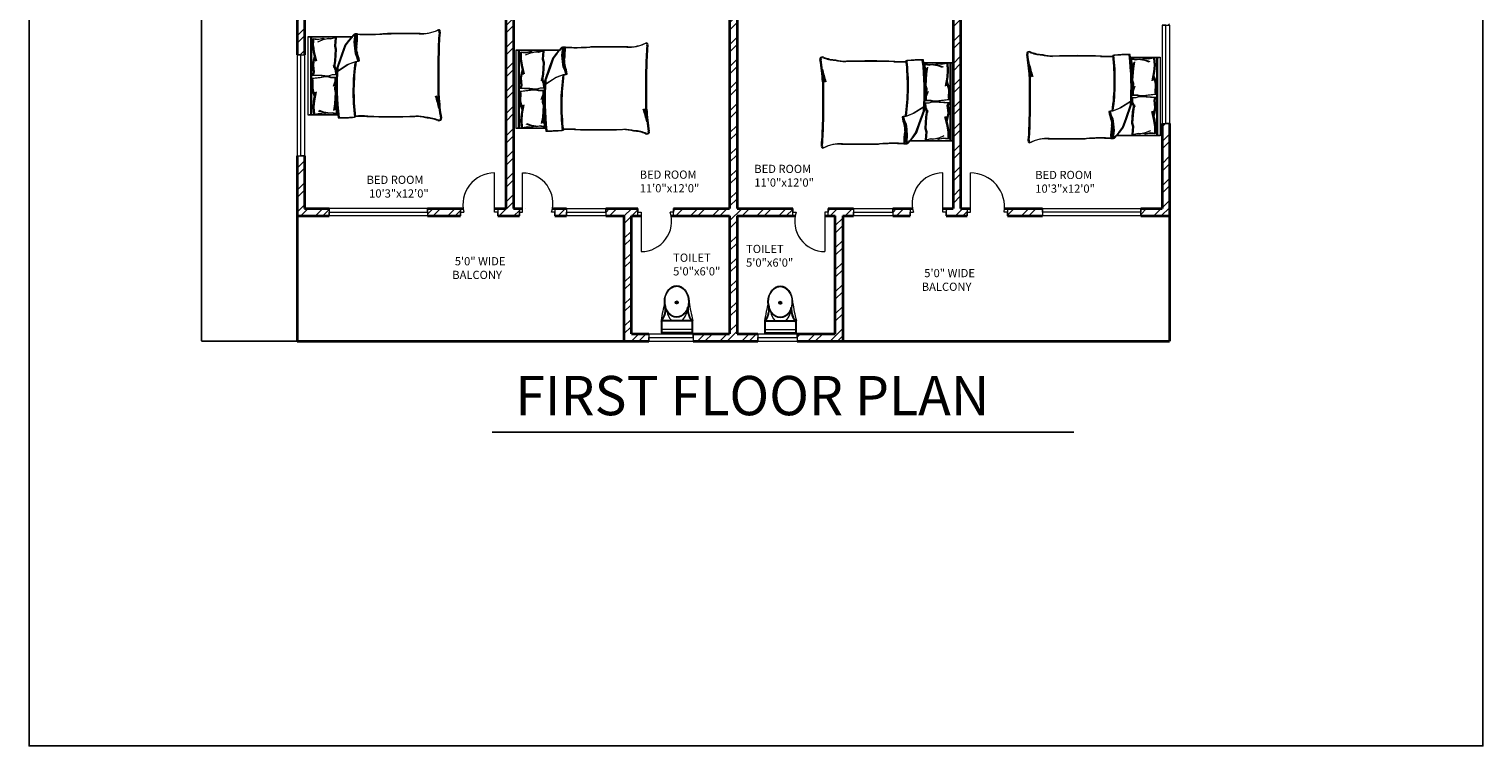
# Model space of a CAD drawing. Units: inches. Extents: x 2168 to 3056, y 1130 to 2629.
# Tile 1 of 42: x 2168 to 3056, y 1130 to 1568. Entities that reach past the tile are written whole.
import ezdxf

# ---------------------------------------------------------------- set-up
doc = ezdxf.new("R2010")
doc.units = ezdxf.units.IN
for name, color, linetype, lineweight in [('A-ANNO-DIMS', 2, 'Continuous', 18), ('A-ANNO-TTLB', 7, 'Continuous', 25), ('A-AREA-IDEN', 7, 'Continuous', 18), ('A-DOOR', 21, 'Continuous', 18), ('A-FLOR-FIXT', 9, 'Continuous', 18), ('A-FURN', 8, 'Continuous', 13), ('A-GLAZ', 201, 'Continuous', 18), ('A-WALL', 7, 'Continuous', 35)]:
    doc.layers.add(name, color=color, linetype=linetype, lineweight=lineweight)
doc.layers.add('A-WALL-PATT', color=143, linetype='Continuous', lineweight=13, true_color=0x7aafdf)
doc.styles.get("Standard").update_dxf_attribs({"font": 'arial.ttf'})
doc.dimstyles.get("Standard").update_dxf_attribs({"dimtxt": 0.18, "dimasz": 0.18, "dimexe": 0.18, "dimexo": 0.0625, "dimgap": 0.09, "dimtad": 0, "dimtih": 1, "dimtoh": 1, "dimdec": 4, "dimzin": 0, "dimdsep": 46, "dimtxsty": 'Standard', "dimcen": 0.09, "dimadec": 0, "dimazin": 0, "dimtfac": 1, "dimtdec": 4, "dimtofl": 0, "dimtmove": 0, "dimatfit": 3, "dimfxl": 1, "dimtolj": 1, "dimtzin": 0, "dimarcsym": 0})

# ---------------------------------------------------------------- blocks, each defined once
blk = doc.blocks.new('A$C31115884')
for p, q in [((283, 498), (223, 498)), ((258, 466), (258, 523)), ((0, 200), (0, 0)), ((520, 200), (0, 200)), ((510, 54), (0, 54)), ((10, 190), (10, 10)), ((510, 190), (10, 190)), ((10, 10), (510, 10)), ((510, 10), (510, 190)), ((520, 0), (520, 200)), ((0, 0), (520, 0))]:
    blk.add_line(p, q)
blk.add_circle((256, 496), 23.6)
for centre, radius, start, end in [((2778, -205), 2807, 165.4549, 171.7133), ((3237, 905), 2807, 188.2867, 194.5451), ((-295, 403), 365, 324.2091, 9.3499), ((-295, 403), 375, 324.2091, 9.3499), ((384, 406), 293, 190.2774, 224.1564), ((139, 406), 293, 315.8436, 2.6563), ((806, 403), 375, 179.2036, 215.7909), ((806, 403), 365, 170.6501, 215.7909)]:
    blk.add_arc(centre, radius, start, end)
blk.add_ellipse((256, 510), major_axis=(0, -261), ratio=0.772727)
blk.add_open_spline([(256, 259), (263, 259), (270, 260), (288, 262), (299, 265), (320, 273), (330, 278), (350, 291), (360, 299), (378, 316), (386, 326), (402, 347), (409, 358), (421, 383), (427, 395), (436, 422), (440, 436), (445, 465), (447, 480), (448, 509), (448, 524), (445, 553), (443, 568), (436, 596), (432, 610), (422, 636), (416, 649), (402, 672), (395, 683), (379, 703), (370, 712), (351, 728), (341, 735), (321, 746), (310, 751), (289, 757), (278, 759), (256, 761), (245, 761), (223, 757), (212, 754), (191, 746), (181, 741), (161, 728), (151, 720), (133, 703), (125, 693), (110, 672), (103, 660), (90, 636), (85, 623), (76, 596), (72, 582), (67, 553), (66, 538), (64, 509), (65, 494), (68, 465), (70, 450), (77, 422), (81, 408), (91, 382), (97, 370), (111, 346), (118, 335), (135, 316), (144, 307), (162, 291), (172, 284), (193, 273), (203, 269), (225, 262), (236, 260), (250, 259), (253, 259), (256, 259)], degree=3, knots=[0, 0, 0, 0, 0.110105, 0.110105, 0.285049, 0.285049, 0.459994, 0.459994, 0.634938, 0.634938, 0.809882, 0.809882, 0.984827, 0.984827, 1.159771, 1.159771, 1.334715, 1.334715, 1.50966, 1.50966, 1.684604, 1.684604, 1.859549, 1.859549, 2.034493, 2.034493, 2.209437, 2.209437, 2.384382, 2.384382, 2.559326, 2.559326, 2.73427, 2.73427, 2.909215, 2.909215, 3.084159, 3.084159, 3.259103, 3.259103, 3.434048, 3.434048, 3.608992, 3.608992, 3.783936, 3.783936, 3.958881, 3.958881, 4.133825, 4.133825, 4.30877, 4.30877, 4.483714, 4.483714, 4.658658, 4.658658, 4.833603, 4.833603, 5.008547, 5.008547, 5.183491, 5.183491, 5.358436, 5.358436, 5.53338, 5.53338, 5.708324, 5.708324, 5.883269, 5.883269, 6.058213, 6.058213, 6.233158, 6.233158, 6.283185, 6.283185, 6.283185, 6.283185])
blk = doc.blocks.new('BED-DOUBLE')
for p, q in [((0, 51.49), (0.64, 51.49)), ((0, 3.48), (0, 51.49)), ((0, 51.27), (26.61, 51.27)), ((0, 51.27), (26.61, 51.27)), ((0.64, 51.49), (27.25, 51.49)), ((0.64, 51.49), (27.25, 51.49)), ((1.53, 3.48), (1.53, 51.27)), ((1.53, 3.48), (1.53, 51.27)), ((2.17, 3.7), (2.17, 51.49)), ((2.17, 3.7), (2.17, 51.49)), ((2.56, 50.11), (2.46, 44.71)), ((2.56, 50.11), (2.46, 44.71)), ((2.46, 44.71), (2.54, 45.71)), ((2.46, 44.71), (2.54, 45.71)), ((2.54, 45.71), (3.07, 41.91)), ((2.54, 45.71), (3.07, 41.91)), ((2.56, 50.11), (5.77, 49.73)), ((2.56, 50.11), (5.77, 49.73)), ((3.2, 50.34), (3.1, 44.94)), ((3.2, 50.34), (3.1, 44.94)), ((3.1, 44.94), (3.18, 45.94)), ((3.1, 44.94), (3.18, 45.94)), ((3.18, 45.94), (3.71, 42.14)), ((3.18, 45.94), (3.71, 42.14)), ((3.2, 50.34), (6.41, 49.96)), ((3.2, 50.34), (6.41, 49.96)), ((8.26, 49.31), (5.58, 48.13)), ((8.26, 49.31), (5.58, 48.13)), ((5.77, 49.73), (8.34, 50.33)), ((5.77, 49.73), (8.34, 50.33)), ((8.9, 49.54), (6.22, 48.36)), ((8.9, 49.54), (6.22, 48.36)), ((6.41, 49.96), (8.98, 50.56)), ((6.41, 49.96), (8.98, 50.56)), ((11.83, 50.11), (8.26, 49.31)), ((11.83, 50.11), (8.26, 49.31)), ((8.34, 50.33), (9.38, 49.81)), ((8.34, 50.33), (9.38, 49.81)), ((12.47, 50.34), (8.9, 49.54)), ((12.47, 50.34), (8.9, 49.54)), ((8.98, 50.56), (10.02, 50.04)), ((8.98, 50.56), (10.02, 50.04)), ((13.43, 49.92), (11.83, 50.11)), ((13.43, 49.92), (11.83, 50.11)), ((14.07, 50.15), (12.47, 50.34)), ((14.07, 50.15), (12.47, 50.34)), ((16.57, 50.7), (13.43, 49.92)), ((16.57, 50.7), (13.43, 49.92)), ((17.21, 50.93), (14.07, 50.15)), ((17.21, 50.93), (14.07, 50.15)), ((16.17, 45.57), (16.57, 50.7)), ((16.17, 45.57), (16.57, 50.7)), ((16.73, 43.61), (16.17, 45.57)), ((16.73, 43.61), (16.17, 45.57)), ((16.81, 45.8), (17.21, 50.93)), ((16.81, 45.79), (17.21, 50.93)), ((17.37, 43.83), (16.81, 45.8)), ((17.37, 43.83), (16.81, 45.79)), ((22.33, 46.22), (20.32, 40.64)), ((22.33, 46.22), (20.32, 40.64)), ((22.97, 46.45), (20.96, 40.87)), ((22.97, 46.45), (20.96, 40.87)), ((24.5, 49.16), (22.33, 46.22)), ((24.5, 49.16), (22.33, 46.22)), ((25.14, 49.39), (22.97, 46.45)), ((25.14, 49.39), (22.97, 46.45)), ((27.75, 52.87), (24.5, 49.16)), ((27.75, 52.87), (24.5, 49.16)), ((28.39, 53.1), (25.14, 49.39)), ((28.39, 53.1), (25.14, 49.39)), ((29.49, 52.95), (27.75, 52.87, 3.87)), ((29.49, 52.95), (27.75, 52.87, 3.87)), ((28.37, 51.33), (27.75, 52.87)), ((28.37, 51.33), (27.75, 52.87)), ((28.06, 48.23), (28.37, 51.33)), ((28.06, 48.23), (28.37, 51.33)), ((28.37, 44.36), (28.06, 48.23)), ((28.37, 44.36), (28.06, 48.23)), ((30.13, 53.18), (28.39, 53.1, 3.87)), ((30.13, 53.18), (28.39, 53.1, 3.87)), ((29, 51.56), (28.39, 53.1)), ((29, 51.56), (28.39, 53.1)), ((28.7, 48.46), (29, 51.56)), ((28.7, 48.46), (29, 51.56)), ((29, 44.59), (28.7, 48.46)), ((29, 44.59), (28.7, 48.46)), ((29.47, 41.18), (29, 44.59)), ((29.47, 41.18), (29, 44.59)), ((3.08, 37.14), (2.54, 34.2)), ((3.08, 37.14), (2.54, 34.2)), ((3.07, 41.91), (4.42, 36.5)), ((3.07, 41.91), (4.42, 36.49)), ((3.67, 39.2), (3.08, 37.14)), ((3.67, 39.2), (3.08, 37.14)), ((3.72, 37.36), (3.18, 34.43)), ((3.72, 37.36), (3.18, 34.43)), ((3.71, 42.14), (5.06, 36.72)), ((3.71, 42.14), (5.06, 36.72)), ((4.31, 39.43), (3.72, 37.36)), ((4.31, 39.43), (3.72, 37.36)), ((15.63, 32.56), (16.3, 36.6)), ((15.63, 32.56), (16.3, 36.6)), ((16.27, 32.79), (16.93, 36.82)), ((16.27, 32.79), (16.93, 36.82)), ((16.3, 36.6), (16.73, 43.61)), ((16.3, 36.6), (16.73, 43.61)), ((16.93, 36.82), (17.37, 43.83)), ((16.93, 36.82), (17.37, 43.83)), ((20.32, 40.64), (17.38, 32.31)), ((20.32, 40.64), (17.38, 32.31)), ((20.96, 40.87), (18.02, 32.53)), ((20.96, 40.87), (18.02, 32.53)), ((23.88, 34.45), (28.37, 36.15)), ((23.88, 34.45), (28.37, 36.15)), ((24.52, 34.68), (29, 36.38)), ((24.52, 34.68), (29, 36.38)), ((28.83, 40.95), (28.37, 44.36)), ((28.83, 40.95), (28.37, 44.36)), ((28.37, 36.15), (30.38, 36.46)), ((28.37, 36.15), (30.38, 36.46)), ((29.76, 38.94), (28.83, 40.95)), ((29.76, 38.94), (28.83, 40.95)), ((29, 36.38), (31.02, 36.69)), ((29, 36.38), (31.02, 36.69)), ((30.4, 39.17), (29.47, 41.18)), ((30.4, 39.17), (29.47, 41.18)), ((30.38, 36.46), (29.76, 38.94)), ((30.38, 36.46), (29.76, 38.94)), ((31.02, 36.69), (30.4, 39.17)), ((31.02, 36.69), (30.4, 39.17)), ((79.25, 15.06), (79.25, 39.68)), ((79.25, 15.06), (79.25, 39.68)), ((79.88, 15.29), (79.88, 39.91)), ((79.88, 15.29), (79.88, 39.91)), ((2.98, 29.46), (2.49, 27.98)), ((2.98, 29.46), (2.49, 27.98)), ((2.49, 27.98), (7.87, 27.73)), ((2.49, 27.98), (7.87, 27.73)), ((2.51, 26.21), (7.86, 26.79)), ((2.51, 26.21), (7.86, 26.79)), ((2.54, 34.2), (2.56, 33.88)), ((2.54, 34.2), (2.56, 33.88)), ((2.56, 33.88), (2.98, 29.46)), ((2.56, 33.88), (2.98, 29.46)), ((3.62, 29.68), (3.13, 28.21)), ((3.62, 29.68), (3.13, 28.21)), ((3.13, 28.21), (8.51, 27.96)), ((3.13, 28.21), (8.51, 27.96)), ((3.18, 34.43), (3.2, 34.11)), ((3.18, 34.43), (3.2, 34.11)), ((3.2, 34.11), (3.62, 29.68)), ((3.2, 34.11), (3.62, 29.68)), ((7.22, 26.56), (10.4, 27.14)), ((7.22, 26.56), (10.4, 27.14)), ((7.86, 26.79), (11.04, 27.37)), ((7.86, 26.79), (11.04, 27.37)), ((7.87, 27.73), (11.08, 27.36)), ((7.87, 27.73), (11.08, 27.35)), ((8.51, 27.96), (11.72, 27.58)), ((8.51, 27.96), (11.72, 27.58)), ((10.4, 27.14), (11.7, 27.14)), ((10.4, 27.14), (11.7, 27.14)), ((11.04, 27.37), (12.34, 27.37)), ((11.04, 27.37), (12.34, 27.37)), ((11.08, 27.36), (12.38, 27.44)), ((11.08, 27.35), (12.38, 27.44)), ((11.7, 27.14), (13.58, 26.56)), ((11.7, 27.14), (13.58, 26.56)), ((11.72, 27.58), (13.02, 27.66)), ((11.72, 27.58), (13.02, 27.66)), ((12.34, 27.37), (14.22, 26.79)), ((12.34, 27.37), (14.22, 26.79)), ((12.38, 27.44), (14.22, 28.13)), ((12.38, 27.44), (14.22, 28.13)), ((13.02, 27.66), (14.86, 28.36)), ((13.02, 27.66), (14.86, 28.36)), ((14.22, 28.13), (16.89, 28.3)), ((14.22, 28.13), (16.89, 28.3)), ((14.22, 26.79), (16.9, 26.79)), ((14.22, 26.79), (16.9, 26.79)), ((14.86, 28.36), (17.53, 28.53)), ((14.86, 28.36), (17.53, 28.53)), ((16.74, 30.75), (15.45, 33.82)), ((16.74, 30.75), (15.45, 33.82)), ((17.38, 30.98), (16.09, 34.05)), ((17.38, 30.98), (16.09, 34.05)), ((16.89, 28.3), (16.74, 30.75)), ((16.89, 28.3), (16.74, 30.75)), ((16.9, 26.79), (16.9, 24.33)), ((16.9, 26.79), (16.9, 24.33)), ((17.38, 30.26), (23.88, 34.45)), ((17.38, 30.26), (23.88, 34.45)), ((17.53, 28.53), (17.38, 30.98)), ((17.53, 28.53), (17.38, 30.98)), ((18.02, 30.49), (24.52, 34.68)), ((18.02, 30.49), (24.52, 34.68)), ((1.87, 25.98), (7.22, 26.56)), ((1.87, 25.98), (7.22, 26.56)), ((2.45, 24.54), (1.87, 25.98)), ((2.45, 24.54), (1.87, 25.98)), ((2.3, 20.09), (2.45, 24.54)), ((2.3, 20.09), (2.45, 24.54)), ((2.3, 19.77), (2.3, 20.09)), ((2.3, 19.77), (2.3, 20.09)), ((3.03, 16.88), (2.3, 19.77)), ((3.03, 16.88), (2.3, 19.77)), ((3.09, 24.77), (2.51, 26.21)), ((3.09, 24.77), (2.51, 26.21)), ((2.94, 20.32), (3.09, 24.77)), ((2.94, 20.32), (3.09, 24.77)), ((2.94, 20), (2.94, 20.32)), ((2.94, 20), (2.94, 20.32)), ((3.67, 17.11), (2.94, 20)), ((3.67, 17.11), (2.94, 20)), ((3.96, 12.34), (4.97, 17.83)), ((3.96, 12.34), (4.97, 17.83)), ((13.58, 26.56), (16.26, 26.56)), ((13.58, 26.56), (16.26, 26.56)), ((16.26, 24.1), (15.17, 20.96)), ((16.26, 24.1), (15.17, 20.96)), ((16.9, 24.33), (15.81, 21.19)), ((16.9, 24.33), (15.81, 21.19)), ((16.17, 19.38), (16.57, 24.52)), ((16.17, 19.38), (16.57, 24.52)), ((16.73, 17.42), (16.17, 19.38)), ((16.73, 17.42), (16.17, 19.38)), ((16.26, 26.56), (16.26, 24.1)), ((16.26, 26.56), (16.26, 24.1)), ((16.81, 19.61), (17.21, 24.74)), ((16.81, 19.61), (17.21, 24.74)), ((17.37, 17.65), (16.81, 19.61)), ((17.37, 17.65), (16.81, 19.61)), ((3.75, 14.86), (3.03, 16.88)), ((3.75, 14.85), (3.03, 16.88)), ((3.03, 8.29), (3.32, 12.11)), ((3.03, 8.28), (3.32, 12.11)), ((3.32, 12.11), (4.33, 17.6)), ((3.32, 12.11), (4.33, 17.6)), ((4.39, 15.08), (3.67, 17.11)), ((4.39, 15.08), (3.67, 17.11)), ((3.67, 8.51), (3.96, 12.34)), ((3.67, 8.51), (3.96, 12.34)), ((15.63, 6.38), (16.3, 10.41)), ((15.63, 6.38), (16.3, 10.41)), ((16.27, 6.61), (16.93, 10.64)), ((16.27, 6.61), (16.93, 10.64)), ((16.3, 10.41), (16.73, 17.42)), ((16.3, 10.41), (16.73, 17.42)), ((16.3, 10.41), (16.62, 9.28)), ((16.3, 10.41), (16.62, 9.28)), ((16.62, 9.28), (17.34, 4.18)), ((16.62, 9.28), (17.34, 4.18)), ((16.93, 10.64), (17.37, 17.65)), ((16.93, 10.64), (17.37, 17.65)), ((16.93, 10.64), (17.26, 9.51)), ((16.93, 10.64), (17.26, 9.51)), ((17.26, 9.51), (17.98, 4.41)), ((17.26, 9.51), (17.98, 4.41)), ((18.11, 3.48), (0, 3.48)), ((18.11, 3.48), (0, 3.48)), ((18.75, 3.7), (0.64, 3.7)), ((18.75, 3.7), (0.64, 3.7)), ((3.01, 8.18), (3.03, 8.29)), ((3.01, 8.18), (3.03, 8.28)), ((3.34, 3.9), (3.01, 8.18)), ((3.34, 3.9), (3.01, 8.18)), ((3.32, 3.89), (6.5, 4.47)), ((3.32, 3.89), (6.5, 4.47)), ((3.65, 8.41), (3.67, 8.51)), ((3.65, 8.41), (3.67, 8.51)), ((3.98, 4.13), (3.65, 8.41)), ((3.98, 4.13), (3.65, 8.41)), ((3.96, 4.12), (7.14, 4.7)), ((3.96, 4.12), (7.14, 4.7)), ((8.96, 5.05), (6.21, 6.06)), ((8.96, 5.05), (6.21, 6.06)), ((6.5, 4.47), (9.1, 4.04)), ((6.5, 4.47), (9.1, 4.04)), ((9.59, 5.28), (6.85, 6.29)), ((9.59, 5.28), (6.85, 6.29)), ((7.14, 4.7), (9.74, 4.27)), ((7.14, 4.7), (9.74, 4.27)), ((12.57, 4.47), (8.96, 5.05)), ((12.57, 4.47), (8.96, 5.05)), ((9.1, 4.04), (10.11, 4.62)), ((9.1, 4.04), (10.11, 4.62)), ((13.21, 4.7), (9.59, 5.28)), ((13.21, 4.7), (9.59, 5.28)), ((9.74, 4.27), (10.75, 4.85)), ((9.74, 4.27), (10.75, 4.85)), ((14.16, 4.76), (12.57, 4.47)), ((14.16, 4.76), (12.57, 4.47)), ((14.8, 4.99), (13.21, 4.7)), ((14.8, 4.99), (13.21, 4.7)), ((17.34, 4.18), (14.16, 4.76)), ((17.34, 4.18), (14.16, 4.76)), ((17.98, 4.41), (14.8, 4.99)), ((17.98, 4.41), (14.8, 4.99))]:
    blk.add_line(p, q)
for centre, radius, start, end in [((36.95, 182.49), 129.5, 266.97912, 273.83645), ((36.95, 182.49), 129.5, 266.97912, 273.83645), ((68.46, -4508.51), 4561.86, 90.00217, 90.28689), ((68.46, -4508.52), 4561.86, 90.00217, 90.28689), ((68.67, 76.16), 23.07, 267.47136, 296.46809), ((68.67, 76.16), 23.07, 267.47136, 296.46809), ((69.31, 76.39), 23.07, 267.47136, 296.46809), ((69.31, 76.39), 23.07, 267.47136, 296.46809), ((78.87, 54.41), 1.1, 332.65876, 86.02002), ((78.87, 54.41), 1.1, 332.65876, 86.02002), ((212.28, 41.15), 133.04, 174.4998, 180.63509), ((212.28, 41.15), 133.04, 174.4998, 180.63509), ((79.51, 54.64), 1.1, 332.65876, 86.02002), ((79.51, 54.64), 1.1, 332.65876, 86.02002), ((212.92, 41.38), 133.04, 174.4998, 180.63509), ((212.92, 41.38), 133.04, 174.4998, 180.63509), ((35.07, 43.74), 6.22, 168.6608, 203.73842), ((35.07, 43.74), 6.22, 168.6608, 203.73842), ((-6.66, 51.33), 36.18, 349.87628, 2.56571), ((-6.66, 51.33), 36.18, 349.87628, 2.56571), ((35.71, 43.97), 6.22, 168.6608, 203.73842), ((35.71, 43.97), 6.22, 168.6608, 203.73842), ((36.32, 182.27), 129.5, 266.97912, 273.83645), ((36.32, 182.27), 129.5, 266.97912, 273.83645), ((-6.02, 51.56), 36.18, 349.87628, 2.56571), ((-6.02, 51.56), 36.18, 349.87628, 2.56571), ((67.82, -4508.74), 4561.86, 90.00217, 90.28689), ((67.82, -4508.74), 4561.86, 90.00217, 90.28689), ((156.32, 17.76), 129.02, 171.78449, 186.90062), ((156.32, 17.76), 129.02, 171.78449, 186.90062), ((156.96, 17.98), 129.02, 171.78449, 186.90062), ((156.96, 17.98), 129.02, 171.78449, 186.90062), ((1.48, 31.15), 29.65, 10.66171, 19.88058), ((1.48, 31.15), 29.65, 10.66171, 19.88058), ((2.12, 31.38), 29.65, 10.66171, 19.88058), ((2.12, 31.38), 29.65, 10.66171, 19.88058), ((30.44, 36.64), 0.185, 250.24637, 1.13765), ((30.44, 36.64), 0.185, 250.24637, 1.13765), ((31.08, 36.86), 0.185, 250.24637, 1.13765), ((31.08, 36.86), 0.185, 250.24637, 1.13765), ((182.05, 21.36), 164.97, 176.08655, 186.78213), ((182.05, 21.36), 164.97, 176.08655, 186.78213), ((182.69, 21.59), 164.97, 176.08655, 186.78213), ((182.69, 21.59), 164.97, 176.08655, 186.78213), ((-23.71, -17.22), 106.46, 13.38322, 17.70533), ((-23.71, -17.22), 106.46, 13.38322, 17.70533), ((-23.07, -16.99), 106.46, 13.38322, 17.70533), ((-23.07, -16.99), 106.46, 13.38322, 17.70533), ((200.84, 21.43), 121.76, 182.99578, 189.40907), ((200.84, 21.43), 121.76, 182.99578, 189.40907), ((201.48, 21.66), 121.76, 182.99578, 189.40907), ((201.48, 21.66), 121.76, 182.99578, 189.40907), ((20.1, 85.16), 83.31, 268.72178, 275.60397), ((20.1, 85.16), 83.31, 268.72178, 275.60397), ((20.74, 85.39), 83.31, 268.72178, 275.60397), ((20.74, 85.39), 83.31, 268.72178, 275.60397), ((31.17, -167.31), 170.11, 88.4762, 91.00819), ((31.17, -167.31), 170.11, 88.4762, 91.00819), ((31.81, -167.08), 170.11, 88.4762, 91.00819), ((31.81, -167.08), 170.11, 88.4762, 91.00819), ((50.61, 484.82), 482.31, 268.22771, 271.71854), ((50.61, 484.82), 482.31, 268.22771, 271.71854), ((51.25, 485.05), 482.31, 268.22771, 271.71854), ((51.25, 485.05), 482.31, 268.22771, 271.71854), ((64.52, -26.9), 29.63, 76.06484, 88.91125), ((64.52, -26.9), 29.63, 76.06484, 88.91125), ((65.15, -26.67), 29.63, 76.06484, 88.91125), ((65.15, -26.67), 29.63, 76.06484, 88.91125), ((70.28, -21.66), 23.56, 67.97508, 86.652), ((70.28, -21.66), 23.56, 67.97508, 86.652), ((70.92, -21.43), 23.56, 67.97508, 86.652), ((70.92, -21.43), 23.56, 67.97508, 86.652), ((79.72, 1.09), 1.09, 236.17358, 23.47814), ((79.72, 1.09), 1.09, 236.17358, 23.47814), ((80.36, 1.32), 1.09, 236.17358, 23.47814), ((80.36, 1.32), 1.09, 236.17358, 23.47814)]:
    blk.add_arc(centre, radius, start, end)
blk = doc.blocks.new('WIN-24-OPPOSED-JAMBS')
for p, q in [((0, 4.5), (0, 0)), ((0, 4.5), (24, 4.5)), ((0, 0), (0, 2.25)), ((0, 2.25), (24, 2.25)), ((24, 2.25), (24, 4.5)), ((24, 4.5), (24, 0)), ((0, 0), (24, 0))]:
    blk.add_line(p, q)
blk = doc.blocks.new('WIN-60-OPPOSED-JAMBS')
for p, q in [((2.25, 60), (0, 60)), ((0, 60), (4.5, 60)), ((0, 60), (0, 0)), ((2.25, 0), (2.25, 60)), ((4.5, 60), (4.5, 0)), ((0, 0), (4.5, 0)), ((4.5, 0), (2.25, 0))]:
    blk.add_line(p, q)
blk = doc.blocks.new('WIN-60')
for p, q in [((4.5, 60), (0, 60)), ((0, 0), (0, 60)), ((2.25, 0), (2.25, 60)), ((2.25, 60), (4.5, 60)), ((4.5, 60), (4.5, 0)), ((0, 0), (4.5, 0)), ((4.5, 0), (2.25, 0))]:
    blk.add_line(p, q)
blk = doc.blocks.new('*D41')
at = {"layer": 'A-ANNO-DIMS', "color": 0, "lineweight": -2, "transparency": 16777216}
for p, q in [((2331.73, 2478.39), (2273.32, 2478.39)), ((2273.5, 2478.21), (2273.5, 1928.07)), ((2273.5, 1377.57), (2273.5, 1927.71)), ((2331.73, 1377.39), (2273.32, 1377.39))]:
    blk.add_line(p, q, dxfattribs=at)
at = {"layer": 'A-ANNO-DIMS', "color": 0, "transparency": 16777216}
for points in [[(2273.47, 2478.21), (2273.53, 2478.21), (2273.5, 2478.39)], [(2273.47, 1377.57), (2273.53, 1377.57), (2273.5, 1377.39)]]:
    blk.add_solid(points, dxfattribs=at)
at = {"layer": 'Defpoints', "color": 0, "transparency": 16777216}
for p in [(2273.5, 2478.39), (2331.8, 2478.39), (2331.8, 1377.39)]:
    blk.add_point(p, dxfattribs=at)
at = {"layer": 'A-ANNO-DIMS', "color": 0, "transparency": 16777216, "insert": (2273.5, 1927.89), "char_height": 0.18, "attachment_point": 5}
blk.add_mtext('\\A1;1101', dxfattribs=at)

msp = doc.modelspace()

# ---------------------------------------------------------------- hatches: boundary and pattern name
at = {"layer": 'A-WALL-PATT'}
h = msp.add_hatch(dxfattribs=at)
h.set_pattern_fill('ANSI32', color=256)
h.paths.add_polyline_path([(2463.8, 2409.39), (2467.39, 2409.39), (2467.39, 2413.89), (2454.77, 2413.89), (2454.77, 2411.64), (2454.77, 2409.39), (2459.3, 2409.39), (2459.3, 2265.39), (2455.64, 2265.39), (2455.64, 2260.89), (2467.35, 2260.89), (2467.35, 2263.14), (2467.35, 2265.39), (2463.8, 2265.39)])
h.paths.add_polyline_path([(2431.6, 2413.89), (2409.65, 2413.89), (2409.65, 2409.39), (2431.6, 2409.39), (2431.6, 2411.64)])
h.paths.add_polyline_path([(2349.65, 2413.89), (2331.8, 2413.89), (2331.8, 2362.67), (2336.3, 2362.67), (2336.3, 2409.39), (2349.65, 2409.39), (2349.65, 2411.64)])
h.paths.add_polyline_path([(2634.15, 2411.64), (2634.15, 2413.89), (2562.29, 2413.89), (2562.29, 2409.39), (2595.8, 2409.39), (2595.8, 2280.31), (2595.83, 2280.31), (2595.83, 2265.39), (2499.91, 2265.39), (2499.91, 2260.89), (2550.8, 2260.89), (2550.8, 2117.31), (2555.3, 2117.31), (2555.3, 2168.08), (2571.93, 2168.08), (2571.93, 2176.89), (2559.8, 2176.89), (2559.8, 2256.39), (2640.8, 2256.39), (2640.8, 2176.89), (2626.43, 2176.89), (2626.43, 2168.08), (2645.3, 2168.08), (2645.3, 2116.64), (2649.8, 2116.64), (2649.8, 2260.89), (2691.25, 2260.89), (2691.25, 2263.14), (2691.25, 2265.39), (2670.65, 2265.39), (2670.65, 2265.36), (2600.3, 2265.36), (2600.3, 2280.26), (2600.3, 2409.39), (2634.15, 2409.39)])
h.paths.add_polyline_path([(2600.3, 2473.89), (2612.84, 2473.89), (2612.84, 2478.39), (2572.64, 2478.39), (2572.64, 2473.89), (2595.8, 2473.89), (2595.8, 2413.89), (2600.3, 2413.89)])
h.paths.add_polyline_path([(2535.8, 2473.89), (2548.64, 2473.89), (2548.64, 2478.39), (2531.4, 2478.39), (2531.4, 2413.89), (2521.6, 2413.89), (2521.6, 2409.39), (2539.24, 2409.39), (2539.24, 2411.64), (2539.24, 2413.89), (2535.8, 2413.89)])
h.paths.add_polyline_path([(2664.8, 2478.39), (2636.84, 2478.39), (2636.84, 2473.89), (2660.3, 2473.89), (2660.3, 2413.89), (2656.17, 2413.89), (2656.17, 2409.39), (2671.68, 2409.39), (2671.68, 2411.64), (2671.68, 2413.89), (2664.8, 2413.89)])
h.paths.add_polyline_path([(2705.94, 2413.89), (2695.68, 2413.89), (2695.68, 2409.39), (2705.94, 2409.39)])
h.paths.add_polyline_path([(2741.35, 2413.89), (2728.73, 2413.89), (2728.73, 2411.64), (2728.73, 2409.39), (2732.3, 2409.39), (2732.3, 2265.39), (2725.73, 2265.39), (2725.73, 2260.89), (2740.92, 2260.89), (2740.92, 2263.14), (2740.92, 2265.39), (2736.8, 2265.39), (2736.8, 2409.39), (2741.35, 2409.39)])
h.paths.add_polyline_path([(2785.65, 2413.89), (2764.55, 2413.89), (2764.49, 2409.39), (2785.65, 2409.39), (2785.65, 2411.64)])
h.paths.add_polyline_path([(2864.3, 2413.89), (2845.65, 2413.89), (2845.65, 2409.39), (2859.8, 2409.39), (2859.8, 2368.43), (2864.3, 2368.43)])
h.paths.add_polyline_path([(2864.3, 2308.43), (2862.05, 2308.43), (2859.8, 2308.43), (2859.8, 2265.39), (2774.48, 2265.39), (2774.48, 2263.14), (2774.48, 2260.89), (2781.8, 2260.89), (2781.8, 2226.65), (2786.3, 2226.65), (2786.3, 2260.89), (2859.8, 2260.89), (2859.8, 2241.35), (2864.3, 2241.35)])
h.paths.add_polyline_path([(2864.3, 2217.35), (2862.05, 2217.35), (2859.8, 2217.35), (2859.8, 2200.89), (2786.3, 2200.89), (2786.3, 2205.93), (2784.05, 2205.93), (2781.8, 2205.93), (2781.8, 2150.97), (2786.3, 2150.97), (2786.3, 2161.89), (2859.8, 2161.89), (2859.8, 2144.42), (2864.3, 2144.42)])
h.paths.add_polyline_path([(2859.8, 2196.39), (2859.8, 2166.39), (2786.3, 2166.39), (2786.3, 2196.39)], flags=16)
h.paths.add_polyline_path([(2864.3, 2108.42), (2862.05, 2108.42), (2859.8, 2108.42), (2859.8, 2080.89), (2786.3, 2080.89), (2786.3, 2111.99), (2781.8, 2111.99), (2781.8, 2080.89), (2649.8, 2080.89), (2649.8, 2086.04), (2647.55, 2086.04), (2645.3, 2086.04), (2645.3, 2071.74), (2649.8, 2071.74), (2649.8, 2076.39), (2781.8, 2076.39), (2781.8, 2041.79), (2786.3, 2041.79), (2786.3, 2076.39), (2859.8, 2076.39), (2859.8, 2058.58), (2864.3, 2058.58)])
h.paths.add_polyline_path([(2864.3, 2022.58), (2859.8, 2022.58), (2859.8, 1992.39), (2786.3, 1992.39), (2786.3, 1999.57), (2781.8, 1999.57), (2781.8, 1848.09), (2784.05, 1848.09), (2786.3, 1848.09), (2786.3, 1851.39), (2859.8, 1851.39), (2859.8, 1838.26), (2864.3, 1838.26)], flags=17)
h.paths.add_polyline_path([(2859.8, 1987.89), (2859.8, 1855.89), (2786.3, 1855.89), (2786.3, 1987.89)], flags=16)
h.paths.add_polyline_path([(2823.05, 1987.89), (2841.42, 1921.89), (2823.05, 1855.89)], flags=0)
h.paths.add_polyline_path([(2864.3, 1814.26), (2859.8, 1814.26), (2859.8, 1791.39), (2786.3, 1791.39), (2786.3, 1825.66), (2784.05, 1825.66), (2781.8, 1825.66), (2781.8, 1791.39), (2720.15, 1791.39), (2720.15, 1791.27), (2649.8, 1791.27), (2649.8, 1806.16), (2649.8, 2038.98), (2647.55, 2038.98), (2645.3, 2038.98), (2645.3, 1783.93), (2649.8, 1783.93), (2649.8, 1786.89), (2781.8, 1786.89), (2781.8, 1746.79), (2786.3, 1746.79), (2786.3, 1786.89), (2859.8, 1786.89), (2859.8, 1770.08), (2864.3, 1770.08)])
h.paths.add_polyline_path([(2864.3, 1734.08), (2862.05, 1734.08), (2859.8, 1734.08), (2859.8, 1705.89), (2786.3, 1705.89), (2786.3, 1714.17), (2781.8, 1714.17), (2781.8, 1660.53), (2786.3, 1660.53), (2786.3, 1666.89), (2859.8, 1666.89), (2859.8, 1648.34), (2864.3, 1648.34)])
h.paths.add_polyline_path([(2786.3, 1701.39), (2859.8, 1701.39), (2859.8, 1671.39), (2786.3, 1671.39)], flags=16)
h.paths.add_polyline_path([(2649.8, 1756.58), (2647.55, 1756.58), (2645.3, 1756.58), (2645.3, 1606.89), (2555.3, 1606.89), (2555.3, 1749.51), (2553.05, 1749.51), (2550.8, 1749.51), (2550.8, 1606.89), (2503.01, 1606.89), (2503.01, 1604.64), (2503.01, 1602.39), (2595.8, 1602.39), (2595.85, 1602.39), (2595.85, 1587.5), (2595.8, 1458.39), (2561.5, 1458.39), (2561.5, 1456.14), (2561.5, 1453.89), (2595.8, 1453.89), (2595.8, 1381.89), (2573.44, 1381.89), (2573.44, 1377.39), (2613.01, 1377.39), (2613.01, 1379.64), (2613.01, 1381.89), (2600.3, 1381.89), (2600.3, 1453.89), (2634.33, 1453.89), (2634.33, 1458.39), (2600.3, 1458.39), (2600.3, 1602.39), (2670.65, 1602.39), (2694.09, 1602.39), (2694.09, 1606.89), (2649.8, 1606.89)])
h.paths.add_polyline_path([(2736.8, 1602.39), (2741.56, 1602.39), (2741.56, 1606.89), (2726.2, 1606.89), (2726.2, 1604.64), (2726.2, 1602.39), (2732.3, 1602.39), (2732.3, 1458.39), (2727.9, 1458.39), (2727.9, 1453.89), (2740.82, 1453.89), (2740.82, 1456.14), (2740.82, 1458.39), (2736.8, 1458.39)])
h.paths.add_polyline_path([(2859.8, 1606.89), (2786.3, 1606.89), (2786.3, 1637.33), (2784.05, 1637.33), (2781.8, 1637.33), (2781.8, 1606.89), (2775.61, 1606.89), (2775.61, 1602.39), (2859.8, 1602.39)])
h.paths.add_polyline_path([(2864.3, 1624.34), (2862.05, 1624.34), (2859.8, 1624.34), (2859.8, 1570.39), (2864.3, 1570.39)])
h.paths.add_polyline_path([(2864.3, 1510.39), (2862.05, 1510.39), (2859.8, 1510.39), (2859.8, 1458.39), (2846.73, 1458.39), (2846.73, 1456.14), (2846.73, 1453.89), (2864.3, 1453.89)])
h.paths.add_polyline_path([(2786.73, 1458.39), (2765.44, 1458.39), (2765.44, 1453.89), (2786.73, 1453.89)])
h.paths.add_polyline_path([(2706, 1458.39), (2695.36, 1458.39), (2695.36, 1453.89), (2706, 1453.89), (2706, 1456.14)])
h.paths.add_polyline_path([(2671.36, 1456.14), (2671.36, 1458.39), (2655.99, 1458.39), (2655.99, 1456.14), (2655.99, 1453.89), (2660.3, 1453.89), (2660.3, 1381.89), (2637.01, 1381.89), (2637.01, 1377.39), (2664.8, 1377.39), (2664.8, 1453.89), (2671.36, 1453.89)], flags=17)
h.paths.add_polyline_path([(2539.83, 1458.39), (2520.24, 1458.39), (2520.24, 1453.89), (2531.3, 1453.89), (2531.3, 1377.39), (2546.45, 1377.39), (2546.45, 1379.64), (2546.45, 1381.89), (2535.8, 1381.89), (2535.8, 1453.89), (2539.83, 1453.89)], flags=17)
h.paths.add_polyline_path([(2496.24, 1458.39), (2489.13, 1458.39), (2489.13, 1453.89), (2496.24, 1453.89), (2496.24, 1456.14)])
h.paths.add_polyline_path([(2467.43, 1456.14), (2467.43, 1458.39), (2463.8, 1458.39), (2463.8, 1602.39), (2468.24, 1602.39), (2468.24, 1605.7), (2468.24, 1606.89), (2454.6, 1606.89), (2454.6, 1602.39), (2459.3, 1602.39), (2459.3, 1458.39), (2454.24, 1458.39), (2454.24, 1453.89), (2467.43, 1453.89)])
h.paths.add_polyline_path([(2431.6, 1456.14), (2431.6, 1458.39), (2411.39, 1458.39), (2411.39, 1453.89), (2431.6, 1453.89)])
h.paths.add_polyline_path([(2351.39, 1458.39), (2336.3, 1458.39), (2336.3, 1490.69), (2334.05, 1490.69), (2331.8, 1490.69), (2331.8, 1453.89), (2351.39, 1453.89), (2351.39, 1456.14)])
h.paths.add_polyline_path([(2336.3, 1629.7), (2331.8, 1629.7), (2331.8, 1552.32), (2336.3, 1552.32), (2336.3, 1602.39), (2406.65, 1602.39), (2423.47, 1602.39), (2423.47, 1606.89), (2418.8, 1606.89), (2418.8, 1643.68), (2416.55, 1643.68), (2414.3, 1643.68), (2414.3, 1606.89), (2336.3, 1606.89)])
h.paths.add_polyline_path([(2418.8, 1714.38), (2414.3, 1714.38), (2414.3, 1705.89), (2336.3, 1705.89), (2336.3, 1731.32), (2334.05, 1731.32), (2331.8, 1731.32), (2331.8, 1653.7), (2334.05, 1653.7), (2336.3, 1653.7), (2336.3, 1666.89), (2414.3, 1666.89), (2414.3, 1663.59), (2418.8, 1663.59)])
h.paths.add_polyline_path([(2336.3, 1701.39), (2414.3, 1701.39), (2414.3, 1671.39), (2336.3, 1671.39)], flags=16)
h.paths.add_polyline_path([(2555.3, 2040.06), (2550.8, 2040.06), (2550.8, 1791.39), (2550.56, 1791.2), (2480.2, 1791.2), (2418.8, 1791.39), (2418.8, 1825.45), (2416.55, 1825.45), (2414.3, 1825.45), (2414.3, 1791.39), (2336.3, 1791.39), (2336.3, 1806.41), (2331.8, 1806.41), (2331.8, 1767.32), (2336.3, 1767.32), (2336.3, 1786.89), (2414.3, 1786.89), (2414.3, 1745.46), (2418.8, 1745.46), (2418.8, 1786.89), (2550.8, 1786.89), (2550.8, 1783.01), (2555.3, 1783.01)])
h.paths.add_polyline_path([(2418.8, 1923.39), (2423.21, 1923.39), (2423.21, 1925.64), (2423.21, 1927.89), (2418.8, 1927.89), (2418.8, 2000.05), (2414.3, 2000.05), (2414.3, 1992.39), (2336.3, 1992.39), (2336.3, 1987.89), (2414.3, 1987.89), (2414.3, 1855.89), (2336.3, 1855.89), (2336.3, 1851.39), (2414.3, 1851.39), (2414.3, 1846.76), (2418.8, 1846.76)], flags=17)
h.paths.add_polyline_path([(2336.3, 2019.29), (2334.05, 2019.29), (2331.8, 2019.29), (2331.8, 1830.41), (2336.3, 1830.41)], flags=17)
h.paths.add_polyline_path([(2550.8, 1927.89), (2453.54, 1927.89), (2453.54, 1925.64), (2453.54, 1923.39), (2550.8, 1923.39)], flags=17)
h.paths.add_polyline_path([(2744.99, 1927.89), (2649.8, 1927.89), (2649.8, 1923.39), (2744.99, 1923.39), (2744.99, 1925.64)], flags=17)
h.paths.add_polyline_path([(2555.3, 2086.46), (2553.05, 2086.46), (2550.8, 2086.46), (2550.8, 2080.89), (2418.8, 2080.89), (2336.3, 2080.89), (2336.3, 2115.4), (2334.05, 2115.4), (2331.8, 2115.4), (2331.8, 2055.29), (2336.3, 2055.29), (2336.3, 2076.39), (2550.8, 2076.39), (2550.8, 2071.54), (2555.3, 2071.54)])
h.paths.add_polyline_path([(2418.8, 2121.39), (2414.3, 2121.39), (2414.3, 2080.89), (2418.8, 2080.89)])
h.paths.add_polyline_path([(2418.8, 2076.39), (2414.3, 2076.39), (2414.3, 2035.12), (2418.8, 2035.12)])
h.paths.add_polyline_path([(2422.87, 2263.14), (2422.87, 2265.39), (2406.65, 2265.39), (2406.65, 2265.36), (2336.3, 2265.36), (2336.3, 2280.25), (2336.3, 2302.67), (2334.05, 2302.67), (2331.8, 2302.67), (2331.8, 2246.85), (2336.3, 2246.85), (2336.3, 2260.89), (2414.3, 2260.89), (2414.3, 2224), (2418.8, 2224), (2418.8, 2260.89), (2422.87, 2260.89)])
h.paths.add_polyline_path([(2418.8, 2204.78), (2416.55, 2204.78), (2414.3, 2204.78), (2414.3, 2200.89), (2336.3, 2200.89), (2336.3, 2220.85), (2331.8, 2220.85), (2331.8, 2151.4), (2336.3, 2151.4), (2336.3, 2161.89), (2414.3, 2161.89), (2414.3, 2153.73), (2418.8, 2153.73)])
h.paths.add_polyline_path([(2414.3, 2196.39), (2414.3, 2166.39), (2336.3, 2166.39), (2336.3, 2196.39)], flags=16)
h.paths.add_polyline_path([(2375.3, 2181.39), (2336.3, 2166.39), (2336.3, 2196.39)], flags=0)
h.paths.add_polyline_path([(2809.6, 2172.34), (2838.8, 2172.34), (2838.8, 2191), (2809.6, 2191)], flags=8)
h.paths.add_polyline_path([(2849.75, 1919.59), (2849.75, 1952.67), (2831.09, 1952.67), (2831.09, 1919.59)], flags=8)
h.paths.add_polyline_path([(2808.87, 1901.97), (2808.87, 1937.85), (2790.15, 1937.85), (2790.15, 1901.97)], flags=8)
h.paths.add_polyline_path([(2806.28, 1671.9), (2835.49, 1671.9), (2835.49, 1690.55), (2806.28, 1690.55)], flags=8)
h.paths.add_polyline_path([(2353.19, 1676.55), (2382.39, 1676.55), (2382.39, 1695.21), (2353.19, 1695.21)], flags=8)
h.paths.add_polyline_path([(2360.08, 1832.31), (2389.24, 1832.31), (2389.24, 1850.97), (2360.08, 1850.97)], flags=25)
h.paths.add_polyline_path([(2354.82, 2167.82), (2384.03, 2167.82), (2384.03, 2186.48), (2354.82, 2186.48)], flags=8)

# ---------------------------------------------------------------- linework, layer by layer
at = {"layer": 'A-ANNO-TTLB'}
msp.add_line((2450.92, 1321.9), (2805.88, 1321.9), dxfattribs=at)
msp.add_lwpolyline([(2168.16, 2629.19), (3055.63, 2629.19), (3055.63, 1130.19), (2168.16, 1130.19)], close=True, dxfattribs=at)
at = {"layer": 'A-DOOR'}
for p, q in [((2452.24, 1456.14), (2452.24, 1480.14)), ((2469.43, 1456.14), (2469.43, 1480.14)), ((2725.9, 1456.14), (2725.9, 1480.14)), ((2742.82, 1456.14), (2742.82, 1480.14)), ((2431.6, 1458.39), (2431.6, 1453.89)), ((2431.6, 1453.89), (2431.6, 1456.14)), ((2431.6, 1456.14), (2433.6, 1456.14)), ((2454.24, 1456.14), (2452.24, 1456.14)), ((2454.24, 1458.39), (2454.24, 1453.89)), ((2454.24, 1453.89), (2454.24, 1456.14)), ((2467.43, 1458.39), (2467.43, 1453.89)), ((2467.43, 1453.89), (2467.43, 1456.14)), ((2467.43, 1456.14), (2469.43, 1456.14)), ((2489.13, 1456.14), (2487.13, 1456.14)), ((2489.13, 1458.39), (2489.13, 1453.89)), ((2489.13, 1453.89), (2489.13, 1456.14)), ((2539.83, 1453.89), (2539.83, 1458.39)), ((2539.83, 1458.39), (2539.83, 1456.14)), ((2539.83, 1456.14), (2541.83, 1456.14)), ((2541.83, 1456.14), (2541.83, 1432.14)), ((2561.5, 1456.14), (2559.5, 1456.14)), ((2561.5, 1453.89), (2561.5, 1458.39)), ((2561.5, 1458.39), (2561.5, 1456.14)), ((2634.33, 1453.89), (2634.33, 1458.39)), ((2634.33, 1458.39), (2634.33, 1456.14)), ((2634.33, 1456.14), (2636.33, 1456.14)), ((2655.99, 1456.14), (2653.99, 1456.14)), ((2653.99, 1456.14), (2653.99, 1432.14)), ((2655.99, 1453.89), (2655.99, 1458.39)), ((2655.99, 1458.39), (2655.99, 1456.14)), ((2706, 1458.39), (2706, 1453.89)), ((2706, 1453.89), (2706, 1456.14)), ((2706, 1456.14), (2708, 1456.14)), ((2727.9, 1456.14), (2725.9, 1456.14)), ((2727.9, 1458.39), (2727.9, 1453.89)), ((2727.9, 1453.89), (2727.9, 1456.14)), ((2740.82, 1458.39), (2740.82, 1453.89)), ((2740.82, 1453.89), (2740.82, 1456.14)), ((2740.82, 1456.14), (2742.82, 1456.14)), ((2765.44, 1456.14), (2763.44, 1456.14)), ((2765.44, 1458.39), (2765.44, 1453.89)), ((2765.44, 1453.89), (2765.44, 1456.14))]:
    msp.add_line(p, q, dxfattribs=at)
for centre, radius, start, end in [((2452.24, 1460.9), 19.24, 90, 194.33047), ((2469.43, 1461.61), 18.52, 342.80836, 90), ((2725.9, 1461.47), 18.67, 90, 196.58203), ((2742.82, 1459.28), 20.86, 351.34519, 90), ((2541.83, 1450.65), 18.51, 270, 17.26464), ((2653.99, 1450.64), 18.5, 162.69155, 270)]:
    msp.add_arc(centre, radius, start, end, dxfattribs=at)
at = {"layer": 'A-GLAZ'}
for p, q in [((2334.05, 1552.32), (2331.8, 1552.32)), ((2331.8, 1552.32), (2336.3, 1552.32)), ((2331.8, 1552.32), (2331.8, 1490.69)), ((2334.05, 1492.32), (2334.05, 1552.32)), ((2336.3, 1552.32), (2336.3, 1490.69)), ((2334.05, 1490.69), (2334.05, 1492.32)), ((2331.8, 1490.69), (2336.3, 1490.69)), ((2336.3, 1490.69), (2334.05, 1490.69)), ((2471.07, 1458.39), (2471.07, 1458.39)), ((2496.24, 1458.39), (2496.24, 1453.89)), ((2496.24, 1458.39), (2520.24, 1458.39)), ((2496.24, 1453.89), (2496.24, 1456.14)), ((2496.24, 1456.14), (2520.24, 1456.14)), ((2520.24, 1456.14), (2520.24, 1458.39)), ((2520.24, 1458.39), (2520.24, 1453.89)), ((2671.36, 1458.39), (2671.36, 1453.89)), ((2671.36, 1458.39), (2696.43, 1458.39)), ((2671.36, 1453.89), (2671.36, 1456.14)), ((2671.36, 1456.14), (2695.36, 1456.14)), ((2695.36, 1456.14), (2695.36, 1458.39)), ((2695.36, 1458.39), (2695.36, 1453.89)), ((2846.73, 1458.39), (2846.73, 1458.39)), ((2520.24, 1453.89), (2495.66, 1453.89)), ((2671.36, 1453.89), (2671.36, 1453.89)), ((2695.36, 1453.89), (2671.36, 1453.89)), ((2546.45, 1381.89), (2546.45, 1377.39)), ((2546.45, 1381.89), (2573.44, 1381.89)), ((2546.45, 1377.39), (2546.45, 1379.64)), ((2546.45, 1379.64), (2549.44, 1379.64)), ((2546.45, 1377.39), (2573.44, 1377.39)), ((2549.44, 1379.64), (2573.44, 1379.64)), ((2573.44, 1379.64), (2573.44, 1381.89)), ((2573.44, 1381.89), (2573.44, 1377.39))]:
    msp.add_line(p, q, dxfattribs=at)
at = {"layer": 'A-WALL'}
for p, q in [((2331.8, 1629.7), (2331.8, 1552.32)), ((2336.3, 1602.39), (2336.3, 1552.32)), ((2459.3, 1458.39), (2459.3, 1602.39)), ((2463.8, 1602.39), (2463.8, 1458.39)), ((2595.8, 1602.39), (2595.8, 1458.39)), ((2600.3, 1602.39), (2600.3, 1458.39)), ((2732.3, 1602.39), (2732.3, 1458.39)), ((2736.8, 1602.39), (2736.8, 1458.39)), ((2859.8, 1510.39), (2859.8, 1458.39)), ((2864.3, 1510.39), (2864.3, 1377.39)), ((2331.8, 1490.69), (2331.8, 1377.39)), ((2336.3, 1490.69), (2336.3, 1458.39)), ((2336.3, 1458.39), (2351.39, 1458.39)), ((2336.3, 1458.39), (2351.39, 1458.39)), ((2411.39, 1458.39), (2433.17, 1458.39)), ((2411.39, 1458.39), (2433.17, 1458.39)), ((2452.24, 1458.39), (2459.3, 1458.39)), ((2452.24, 1458.39), (2459.3, 1458.39)), ((2463.8, 1458.39), (2469.43, 1458.39)), ((2463.8, 1458.39), (2469.43, 1458.39)), ((2487.67, 1458.39), (2496.24, 1458.39)), ((2520.24, 1458.39), (2539.83, 1458.39)), ((2561.5, 1458.39), (2595.8, 1458.39)), ((2600.3, 1458.39), (2634.33, 1458.39)), ((2655.99, 1458.39), (2671.36, 1458.39)), ((2695.36, 1458.39), (2707.48, 1458.39)), ((2725.9, 1458.39), (2732.3, 1458.39)), ((2736.8, 1458.39), (2742.82, 1458.39)), ((2763.66, 1458.39), (2786.73, 1458.39)), ((2846.73, 1458.39), (2859.8, 1458.39)), ((2331.8, 1453.89), (2351.39, 1453.89)), ((2411.39, 1453.89), (2431.6, 1453.89)), ((2454.24, 1453.89), (2467.43, 1453.89)), ((2454.24, 1453.89), (2467.43, 1453.89)), ((2489.13, 1453.89), (2496.24, 1453.89)), ((2520.24, 1453.89), (2531.3, 1453.89)), ((2531.3, 1453.89), (2531.3, 1377.39)), ((2535.8, 1381.89), (2535.8, 1453.89)), ((2535.8, 1453.89), (2541.83, 1453.89)), ((2560.05, 1453.89), (2595.8, 1453.89)), ((2595.8, 1453.89), (2595.8, 1381.89)), ((2600.3, 1453.89), (2600.3, 1381.89)), ((2600.3, 1453.89), (2635.78, 1453.89)), ((2653.99, 1453.89), (2660.3, 1453.89)), ((2660.3, 1381.89), (2660.3, 1453.89)), ((2664.8, 1453.89), (2664.8, 1377.39)), ((2664.8, 1453.89), (2671.36, 1453.89)), ((2695.36, 1453.89), (2706, 1453.89)), ((2727.9, 1453.89), (2740.82, 1453.89)), ((2765.44, 1453.89), (2786.73, 1453.89)), ((2765.44, 1453.89), (2786.73, 1453.89)), ((2846.73, 1453.89), (2864.3, 1453.89)), ((2331.8, 1377.39), (2546.45, 1377.39)), ((2535.8, 1381.89), (2546.45, 1381.89)), ((2573.44, 1381.89), (2595.8, 1381.89)), ((2573.44, 1377.39), (2613.01, 1377.39)), ((2600.3, 1381.89), (2613.01, 1381.89)), ((2637.01, 1381.89), (2660.3, 1381.89)), ((2637.01, 1377.39), (2864.3, 1377.39))]:
    msp.add_line(p, q, dxfattribs=at)

# ---------------------------------------------------------------- block references
at = {"layer": 'A-FLOR-FIXT', "xscale": 0.0372717239612423, "yscale": 0.0372717239612423, "zscale": 0.0372717239612423}
for p in [(2553.94, 1382.59), (2617.15, 1382.39)]:
    msp.add_blockref('A$C31115884', p, dxfattribs=at)
at = {"layer": 'A-FURN'}
for p in [(2338.55, 1511.94), (2465.41, 1503.89)]:
    msp.add_blockref('BED-DOUBLE', p, dxfattribs=at)
at = {"layer": 'A-FURN', "rotation": 180}
for p in [(2858.54, 1554.32), (2732.3, 1551.07)]:
    msp.add_blockref('BED-DOUBLE', p, dxfattribs=at)
at = {"layer": 'A-GLAZ'}
for name, p in [('WIN-60-OPPOSED-JAMBS', (2859.8, 1510.39)), ('WIN-24-OPPOSED-JAMBS', (2613.01, 1377.39))]:
    msp.add_blockref(name, p, dxfattribs=at)
for name, p, rotation in [('WIN-60-OPPOSED-JAMBS', (2351.39, 1458.39), 270), ('WIN-60', (2846.74, 1453.89), 90)]:
    msp.add_blockref(name, p, dxfattribs=dict(at, rotation=rotation))

# ---------------------------------------------------------------- texts
at = {"layer": 'A-ANNO-TTLB', "insert": (2464.88, 1356.18), "char_height": 24, "attachment_point": 1}
msp.add_mtext_dynamic_manual_height_columns('FIRST FLOOR PLAN', width=477.3793, gutter_width=12.5, heights=[0], dxfattribs=at)
at = {"layer": 'A-AREA-IDEN', "char_height": 5, "attachment_point": 1}
for s, width, insert in [('BED ROOM\\P11\'0"x12\'0"', 137.6933, (2610.88, 1485.15)), ('   BED ROOM\\P    10\'3"x12\'0"', 89.6616, (2369.63, 1478.47)), ('BED ROOM\\P11\'0"x12\'0"', 122.9946, (2540.91, 1481.64)), ('BED ROOM\\P10\'3"x12\'0"', 181.9397, (2782.39, 1481.44)), ('        5\'0" WIDE\\P       BALCONY', 124.6038, (2415.8, 1428.74)), ('TOILET\\P5\'0"x6\'0"', 47.1577, (2561.32, 1430.9)), ('TOILET\\P5\'0"x6\'0"', 41.5803, (2605.83, 1436.25)), ('    5\'0" WIDE\\P   BALCONY', 169.8821, (2708.5, 1421.49))]:
    msp.add_mtext_dynamic_manual_height_columns(s, width=width, gutter_width=12.5, heights=[0], dxfattribs=dict(at, insert=insert))

# ---------------------------------------------------------------- dimensions: what is measured, and where the dimension line sits
at = {"layer": 'A-ANNO-DIMS'}
dim = msp.add_linear_dim(base=(2273.5, 2478.39), p1=(2331.8, 1377.39), p2=(2331.8, 2478.39), angle=90, dimstyle='Standard', override={"dimdec": 0, "dimlfac": 1, "dimrnd": 0, "dimzin": 0, "dimdsep": 46, "dimlunit": 2}, dxfattribs=at)
dim.commit()
dim.dimension.update_dxf_attribs({"geometry": '*D41', "text_midpoint": (2273.5, 1927.89)})

doc.saveas('drawing.dxf')
